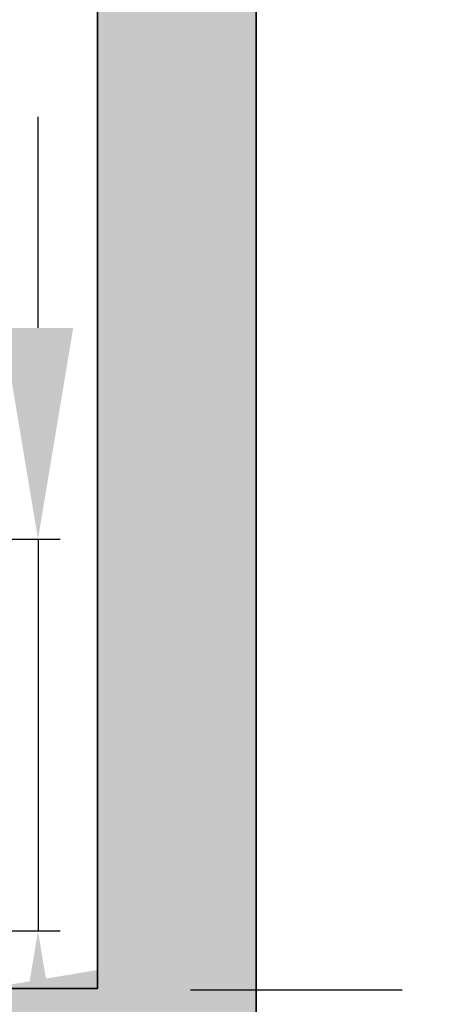
# Model space of a CAD drawing. Units: inches. Extents: x 2083 to 3317, y 1141 to 2115.
# Tile 240 of 256: x 3114 to 3137, y 1271 to 1327. Entities that reach past the tile are written whole.
import ezdxf

# ---------------------------------------------------------------- set-up
doc = ezdxf.new("R2010")
doc.units = ezdxf.units.IN
doc.layers.add('A-ANNO-DIMS', color=2, linetype='Continuous', lineweight=18)
doc.layers.add('A-WALL', color=7, linetype='Continuous', lineweight=35)
doc.layers.add('A-WALL-PATT', color=251, linetype='Continuous', lineweight=13, true_color=0x636466)
doc.styles.get("Standard").update_dxf_attribs({"font": 'arial.ttf'})
doc.dimstyles.new('ISO-25', dxfattribs={"dimtxt": 12, "dimasz": 12, "dimexe": 1.25, "dimexo": 0.625, "dimtad": 1, "dimlunit": 3, "dimtxsty": 'Standard', "dimcen": 2.5, "dimadec": 0, "dimazin": 0, "dimtfac": 1, "dimtmove": 0, "dimatfit": 3, "dimfxl": 1, "dimarcsym": 0})

# ---------------------------------------------------------------- blocks, each defined once
blk = doc.blocks.new('*D9')
at = {"layer": 'A-ANNO-DIMS', "color": 0, "lineweight": -2, "transparency": 16777216}
for p, q in [((3127.585, 1486.761), (3190.403, 1486.761)), ((3189.153, 1474.761), (3189.153, 1275.261)), ((3127.585, 1263.261), (3190.403, 1263.261))]:
    blk.add_line(p, q, dxfattribs=at)
at = {"layer": 'A-ANNO-DIMS', "color": 0, "transparency": 16777216}
for points in [[(3187.153, 1474.761), (3191.153, 1474.761), (3189.153, 1486.761)], [(3187.153, 1275.261), (3191.153, 1275.261), (3189.153, 1263.261)]]:
    blk.add_solid(points, dxfattribs=at)
at = {"layer": 'Defpoints', "color": 0, "transparency": 16777216}
for p in [(3126.96, 1486.761), (3126.96, 1263.261), (3189.153, 1263.261)]:
    blk.add_point(p, dxfattribs=at)
at = {"layer": 'A-ANNO-DIMS', "color": 0, "transparency": 16777216, "insert": (3182.401, 1375.011), "char_height": 12, "attachment_point": 5, "rotation": 90}
blk.add_mtext('18\'-7.5"', dxfattribs=at)
blk = doc.blocks.new('*D26')
at = {"layer": 'A-ANNO-DIMS', "color": 0, "lineweight": -2, "transparency": 16777216}
for p, q in [((3088.986, 1274.915), (3088.986, 1270.952)), ((3111.24, 1274.915), (3111.24, 1270.952)), ((3076.986, 1272.202), (2840.262, 1272.202)), ((3111.24, 1272.202), (3088.986, 1272.202)), ((3123.24, 1272.202), (3135.24, 1272.202))]:
    blk.add_line(p, q, dxfattribs=at)
at = {"layer": 'A-ANNO-DIMS', "color": 0, "transparency": 16777216}
for points in [[(3076.986, 1274.202), (3076.986, 1270.202), (3088.986, 1272.202)], [(3123.24, 1274.202), (3123.24, 1270.202), (3111.24, 1272.202)]]:
    blk.add_solid(points, dxfattribs=at)
at = {"layer": 'Defpoints', "color": 0, "transparency": 16777216}
for p in [(3088.986, 1275.54), (3111.24, 1275.54), (3088.986, 1272.202)]:
    blk.add_point(p, dxfattribs=at)
at = {"layer": 'A-ANNO-DIMS', "color": 0, "transparency": 16777216, "insert": (2952.624, 1279.032), "char_height": 12, "attachment_point": 5}
blk.add_mtext('NIGHTSTAND 1\'-10 1/2" TYP.', dxfattribs=at)
blk = doc.blocks.new('*D27')
at = {"layer": 'A-ANNO-DIMS', "color": 0, "lineweight": -2, "transparency": 16777216}
for p, q in [((3114.578, 1309.794), (3114.578, 1321.794)), ((3111.865, 1297.794), (3115.828, 1297.794)), ((3114.578, 1297.794), (3114.578, 1275.54)), ((3111.865, 1275.54), (3115.828, 1275.54)), ((3114.578, 1263.54), (3114.578, 1140.989))]:
    blk.add_line(p, q, dxfattribs=at)
at = {"layer": 'A-ANNO-DIMS', "color": 0, "transparency": 16777216}
for points in [[(3112.578, 1309.794), (3116.578, 1309.794), (3114.578, 1297.794)], [(3112.578, 1263.54), (3116.578, 1263.54), (3114.578, 1275.54)]]:
    blk.add_solid(points, dxfattribs=at)
at = {"layer": 'Defpoints', "color": 0, "transparency": 16777216}
for p in [(3111.24, 1297.794), (3111.24, 1275.54), (3114.578, 1275.54)]:
    blk.add_point(p, dxfattribs=at)
at = {"layer": 'A-ANNO-DIMS', "color": 0, "transparency": 16777216, "insert": (3107.749, 1196.264), "char_height": 12, "attachment_point": 5, "rotation": 90}
blk.add_mtext('1\'-10 1/2" TYP.', dxfattribs=at)
blk = doc.blocks.new('*D35')
at = {"layer": 'A-ANNO-DIMS', "color": 0, "lineweight": -2, "transparency": 16777216}
for p, q in [((3127.585, 2020.761), (3180.56, 2020.761)), ((3179.31, 1275.261), (3179.31, 2008.761)), ((3127.585, 1263.261), (3180.56, 1263.261))]:
    blk.add_line(p, q, dxfattribs=at)
at = {"layer": 'A-ANNO-DIMS', "color": 0, "transparency": 16777216}
for points in [[(3177.31, 2008.761), (3181.31, 2008.761), (3179.31, 2020.761)], [(3177.31, 1275.261), (3181.31, 1275.261), (3179.31, 1263.261)]]:
    blk.add_solid(points, dxfattribs=at)
at = {"layer": 'Defpoints', "color": 0, "transparency": 16777216}
for p in [(3126.96, 2020.761), (3179.31, 2020.761), (3126.96, 1263.261)]:
    blk.add_point(p, dxfattribs=at)
at = {"layer": 'A-ANNO-DIMS', "color": 0, "transparency": 16777216, "insert": (3172.476, 1642.011), "char_height": 12, "attachment_point": 5, "rotation": 90}
blk.add_mtext('63\'-1 1/2"', dxfattribs=at)

msp = doc.modelspace()

# ---------------------------------------------------------------- hatches: boundary and pattern name
at = {"layer": 'A-WALL-PATT'}
h = msp.add_hatch(color=256, dxfattribs=at)
h.dxf.hatch_style = 1
h.paths.add_polyline_path([(3126.96, 2020.761), (2748.96, 2020.761), (2604.96, 2020.761), (2226.96, 2020.761), (2226.96, 1702.761), (2466.96, 1702.761), (2466.96, 1582.761), (2418.96, 1582.761), (2418.96, 1477.761), (2226.96, 1477.761), (2226.96, 1263.261), (2544.96, 1263.261), (2544.96, 1411.761), (2604.96, 1411.761), (2685.96, 1411.761), (2685.96, 1420.761), (2604.96, 1420.761), (2604.96, 1573.761), (2604.96, 1702.761), (2604.96, 2011.761), (2748.96, 2011.761), (2748.96, 1702.761), (2862.96, 1702.761), (2862.96, 1621.761), (2871.96, 1621.761), (2871.96, 1702.761), (2883.96, 1702.761), (2883.96, 1706.939, -0.026459), (2883.96, 1711.761), (2757.96, 1711.761), (2757.96, 1807.761), (2787.96, 1807.761), (2787.96, 1812.261), (2757.96, 1812.261), (2757.96, 2011.761), (2877.96, 2011.761), (2877.96, 1812.261), (2847.96, 1812.261), (2847.96, 1807.761), (2889.836, 1807.761), (2889.836, 1812.261), (2882.46, 1812.261), (2882.46, 2011.761), (3117.96, 2011.761), (3117.96, 1812.261), (2937.836, 1812.261), (2937.836, 1807.761), (2995.71, 1807.761), (2995.71, 1796.118), (3000.21, 1796.118), (3000.21, 1807.761), (3117.96, 1807.761), (3117.96, 1711.761), (3000.21, 1711.761), (3000.21, 1760.118), (2998.573, 1760.118, -0.020711), (2995.71, 1760.118), (2995.71, 1711.761), (2931.96, 1711.761), (2931.96, 1702.761), (3126.96, 1702.761)])
h.paths.add_polyline_path([(2471.46, 2011.761), (2471.46, 1810.011), (2462.717, 1810.011), (2462.717, 1805.511), (2505.96, 1805.511), (2505.96, 1810.011), (2475.96, 1810.011), (2475.96, 2011.761), (2595.96, 2011.761), (2595.96, 1810.011), (2565.96, 1810.011), (2565.96, 1805.511), (2595.96, 1805.511), (2595.96, 1711.761), (2235.96, 1711.761), (2235.96, 1805.511), (2353.71, 1805.511), (2353.71, 1796.054), (2358.21, 1796.054), (2358.21, 1805.511), (2414.717, 1805.511), (2414.717, 1810.011), (2235.96, 1810.011), (2235.96, 2011.761)], flags=16)
h.paths.add_polyline_path([(2270.205, 1994.61), (2270.205, 1970.61), (2246.205, 1970.61), (2246.205, 1994.61)], flags=0)
edge = h.paths.add_edge_path(flags=0)
edge.add_ellipse((2332.027, 1899.798), major_axis=(-3.043, 3.043), ratio=0.168252, start_angle=-161.3322, end_angle=-156.3071, ccw=False)
edge.add_ellipse((2333.082, 1898.744), major_axis=(-1.055, 1.055), ratio=0.453532, start_angle=-123.371, end_angle=-94.1591)
edge = h.paths.add_edge_path(flags=0)
edge.add_ellipse((2332.027, 1968.876), major_axis=(3.043, 3.043), ratio=0.168252, start_angle=18.6678, end_angle=23.6929)
edge.add_spline(control_points=[(2332.926, 1970.691), (2332.227, 1970.336), (2330.894, 1969.659), (2328.413, 1970.932), (2327.204, 1967.749), (2324.71, 1969.956), (2322.533, 1967.012), (2320.013, 1971.296), (2317.68, 1968.158), (2316.041, 1967.102), (2315.427, 1966.81)], knot_values=[0, 0, 0, 0, 2.267059, 4.324559, 6.685584, 8.878641, 11.121502, 14.300359, 17.755284, 19.732645, 19.732645, 19.732645, 19.732645], degree=3, periodic=0)
edge.add_ellipse((2332.027, 1968.876), major_axis=(3.043, 3.043), ratio=0.168252, start_angle=18.6678, end_angle=23.6929, ccw=False)
edge.add_ellipse((2333.082, 1969.931), major_axis=(1.055, 1.055), ratio=0.453532, start_angle=56.629, end_angle=85.8409, ccw=False)
edge = h.paths.add_edge_path(flags=0)
edge.add_spline(control_points=[(2296.428, 1967.988), (2293.628, 1965.336), (2287.704, 1959.727), (2299.744, 1949.996), (2294.533, 1935.669), (2290.573, 1920.604), (2293.394, 1909.974), (2296.185, 1904.967)], knot_values=[0.099185, 0.099185, 0.099185, 0.099185, 0.345301, 0.619822, 0.982653, 1.386093, 1.810555, 1.810555, 1.810555, 1.810555], degree=3, periodic=0)
edge.add_spline(control_points=[(2296.185, 1904.967), (2297.384, 1902.619), (2298.001, 1901.949), (2298.553, 1901.468)], knot_values=[0.006246, 0.006246, 0.006246, 0.006246, 0.055476, 0.055476, 0.055476, 0.055476], degree=3, periodic=0)
edge.add_spline(control_points=[(2298.553, 1901.468), (2297.259, 1900.923), (2295.225, 1900.232), (2293.06, 1900.614), (2292.101, 1900.788), (2292.09, 1900.791)], knot_values=[0.312835, 0.312835, 0.312835, 0.312835, 0.40178, 0.474987, 0.475903, 0.475903, 0.475903, 0.475903], degree=3, periodic=0)
edge.add_arc((2292.794, 1904.664), 3.937, 215.4209, 259.6982, ccw=False)
edge.add_spline(control_points=[(2289.585, 1902.382), (2289.477, 1902.535), (2289.368, 1902.688), (2289.261, 1902.841)], knot_values=[0.102872, 0.102872, 0.102872, 0.102872, 0.116896, 0.116896, 0.116896, 0.116896], degree=3, periodic=0)
edge.add_spline(control_points=[(2289.261, 1902.841), (2288.687, 1902.55), (2287.64, 1902.02), (2285.881, 1901.874), (2283.853, 1901.504), (2281.72, 1899.711), (2278.467, 1899.493), (2276.157, 1901.883), (2272.259, 1899.804), (2267.778, 1901.843), (2262.244, 1900.184), (2257.415, 1901.782), (2254.318, 1900.726), (2253.178, 1900.337)], knot_values=[0, 0, 0, 0, 1.907977, 3.477176, 5.261074, 7.972851, 11.680248, 13.717921, 16.939592, 22.789562, 27.502503, 33.595215, 37.145618, 37.145618, 37.145618, 37.145618], degree=3, periodic=0)
edge.add_line((2253.178, 1900.337), (2250.244, 1902.841))
edge.add_line((2250.244, 1902.841), (2250.244, 1965.833))
edge.add_line((2250.244, 1965.833), (2253.178, 1968.337))
edge.add_spline(control_points=[(2253.178, 1968.337), (2254.318, 1967.948), (2257.415, 1966.892), (2262.244, 1968.49), (2267.778, 1966.831), (2271.527, 1968.537), (2273.876, 1967.828), (2274.207, 1967.728)], knot_values=[0, 0, 0, 0, 0.09018, 0.244935, 0.364644, 0.513233, 0.537855, 0.537855, 0.537855, 0.537855], degree=3, periodic=0)
edge.add_arc((2274.353, 1963.793), 3.937, 72.0511, 92.1279, ccw=False)
edge.add_arc((2281.297, 1985.23), 18.596, 252.0511, 288.5657)
edge.add_arc((2292.317, 1956.029), 12.646, 71.0268, 113.7782, ccw=False)
edge = h.paths.add_edge_path(flags=0)
edge.add_spline(control_points=[(2274.899, 1951.856), (2275.066, 1951.617), (2275.233, 1951.377), (2275.398, 1951.136)], knot_values=[1.409916, 1.409916, 1.409916, 1.409916, 1.43159, 1.43159, 1.43159, 1.43159], degree=3, periodic=0)
edge.add_spline(control_points=[(2275.398, 1951.136), (2275.792, 1950.562), (2276.179, 1949.984), (2276.546, 1949.397)], knot_values=[1.358238, 1.358238, 1.358238, 1.358238, 1.409916, 1.409916, 1.409916, 1.409916], degree=3, periodic=0)
edge.add_line((2276.546, 1949.397), (2277.437, 1947.862))
edge.add_spline(control_points=[(2277.437, 1947.862), (2276.304, 1945.673), (2274.64, 1942.427), (2274.632, 1938.094), (2272.799, 1930.852), (2274.356, 1943.897), (2275.948, 1947.923), (2276.546, 1949.397)], knot_values=[0.005632, 0.005632, 0.005632, 0.005632, 0.186014, 0.266002, 0.357087, 0.59639, 0.739732, 0.739732, 0.739732, 0.739732], degree=3, periodic=0)
edge.add_spline(control_points=[(2276.546, 1949.397), (2276.179, 1949.984), (2275.792, 1950.562), (2275.398, 1951.136)], knot_values=[1.358238, 1.358238, 1.358238, 1.358238, 1.409916, 1.409916, 1.409916, 1.409916], degree=3, periodic=0)
edge.add_spline(control_points=[(2275.398, 1951.136), (2274.943, 1950.08), (2274.208, 1948.025), (2273.935, 1944.851), (2272.469, 1937.627), (2273.466, 1945.696), (2274.701, 1951.059), (2274.899, 1951.856)], knot_values=[0.104364, 0.104364, 0.104364, 0.104364, 0.189636, 0.269624, 0.36071, 0.600013, 0.644622, 0.644622, 0.644622, 0.644622], degree=3, periodic=0)
h.paths.add_polyline_path([(2269.168, 1963.128, -0.357527), (2268.171, 1960.976, -0.092561), (2268.171, 1939.436, -0.357527), (2269.168, 1937.285, -0.357527), (2267.016, 1938.282, -0.164785), (2254.686, 1938.282, -0.357527), (2252.534, 1937.285, -0.357527), (2253.531, 1939.436, -0.092561), (2253.531, 1960.976, -0.357527), (2252.534, 1963.128, -0.357527), (2254.686, 1962.131, -0.164785), (2267.016, 1962.131, -0.357527)], flags=0)
h.paths.add_polyline_path([(2248.874, 1967.802), (2248.874, 1957.028), (2249.458, 1957.028), (2249.458, 1911.647), (2248.874, 1911.647), (2248.874, 1900.873), (2246.512, 1900.873, 0.197327), (2244.15, 1902.457), (2244.15, 1966.218, 0.197327), (2246.512, 1967.802)], flags=0)
h.paths.add_polyline_path([(2269.168, 1931.389, -0.357527), (2268.171, 1929.238, -0.092561), (2268.171, 1907.698, -0.357527), (2269.168, 1905.547, -0.357527), (2267.016, 1906.544, -0.164785), (2254.686, 1906.544, -0.357527), (2252.534, 1905.547, -0.357527), (2253.531, 1907.698, -0.092561), (2253.531, 1929.238, -0.357527), (2252.534, 1931.389, -0.357527), (2254.686, 1930.392, -0.164785), (2267.016, 1930.392, -0.357527)], flags=0)
edge = h.paths.add_edge_path(flags=0)
edge.add_spline(control_points=[(2276.197, 1906.724), (2276.168, 1909.029), (2276.114, 1913.372), (2270.598, 1924.925), (2273.905, 1919.013), (2275.922, 1916.262), (2275.475, 1912.402), (2277.258, 1910.381), (2276.696, 1908.225), (2276.646, 1906.813), (2276.618, 1906.008)], knot_values=[0, 0, 0, 0, 8.61026, 16.221274, 18.843057, 23.804898, 27.440828, 29.356102, 31.203478, 33.650687, 33.650687, 33.650687, 33.650687], degree=3, periodic=0)
edge.add_spline(control_points=[(2276.618, 1906.008), (2276.623, 1905.624), (2276.498, 1904.629), (2275.442, 1903.855), (2274.937, 1903.08), (2274.859, 1902.841)], knot_values=[0.156488, 0.156488, 0.156488, 0.156488, 0.184398, 0.231376, 0.250598, 0.250598, 0.250598, 0.250598], degree=3, periodic=0)
edge.add_line((2274.859, 1902.841), (2276.506, 1902.841))
edge.add_spline(control_points=[(2276.506, 1902.841), (2276.788, 1903.085), (2277.665, 1904.125), (2278.25, 1904.341), (2277.654, 1908.527), (2278.156, 1906.228), (2278.1, 1905.286), (2278.847, 1904.069), (2277.857, 1903.415), (2277.874, 1902.991), (2277.904, 1902.841)], knot_values=[0.059574, 0.059574, 0.059574, 0.059574, 0.080753, 0.103741, 0.16972, 0.176036, 0.207137, 0.240474, 0.262341, 0.27366, 0.27366, 0.27366, 0.27366], degree=3, periodic=0)
edge.add_line((2277.904, 1902.841), (2280.03, 1902.841))
edge.add_spline(control_points=[(2280.03, 1902.841), (2279.888, 1903.088), (2279.499, 1903.982), (2280.152, 1905.939), (2278.104, 1909.658), (2279.762, 1907.185), (2280.328, 1904.875), (2280.485, 1903.49), (2281.463, 1903.249), (2281.758, 1902.936), (2281.834, 1902.841)], knot_values=[0.013856, 0.013856, 0.013856, 0.013856, 0.034874, 0.088867, 0.107879, 0.126738, 0.158714, 0.193757, 0.217487, 0.226722, 0.226722, 0.226722, 0.226722], degree=3, periodic=0)
edge.add_spline(control_points=[(2281.834, 1902.841), (2281.788, 1902.827), (2281.647, 1902.783), (2281.396, 1902.859), (2281.088, 1902.985), (2280.721, 1903.061), (2280.333, 1903.026), (2280.125, 1902.899), (2280.03, 1902.841)], knot_values=[0, 0, 0, 0, 0.14413, 0.435517, 0.749276, 1.153046, 1.548371, 1.878348, 1.878348, 1.878348, 1.878348], degree=3, periodic=0)
edge.add_line((2280.03, 1902.841), (2277.904, 1902.841))
edge.add_spline(control_points=[(2277.904, 1902.841), (2277.893, 1902.796), (2277.865, 1902.68), (2277.607, 1902.687), (2277.274, 1902.801), (2276.838, 1902.62), (2276.584, 1902.789), (2276.506, 1902.841)], knot_values=[0, 0, 0, 0, 0.127189, 0.326199, 0.628009, 1.24357, 1.515331, 1.515331, 1.515331, 1.515331], degree=3, periodic=0)
edge.add_line((2276.506, 1902.841), (2274.859, 1902.841))
edge.add_spline(control_points=[(2274.859, 1902.841), (2274.814, 1902.899), (2274.725, 1903.013), (2274.493, 1903.119), (2274.244, 1902.961), (2273.937, 1903.185), (2273.614, 1902.983), (2273.408, 1902.883), (2273.322, 1902.841)], knot_values=[0, 0, 0, 0, 0.21843, 0.436957, 0.687977, 0.990379, 1.398396, 1.69185, 1.69185, 1.69185, 1.69185], degree=3, periodic=0)
edge.add_spline(control_points=[(2273.322, 1902.841), (2273.617, 1903.446), (2274.274, 1904.538), (2276.027, 1904.574), (2276.207, 1906.584), (2276.197, 1906.724)], knot_values=[0.012227, 0.012227, 0.012227, 0.012227, 0.059472, 0.106218, 0.134458, 0.134458, 0.134458, 0.134458], degree=3, periodic=0)
h.paths.add_polyline_path([(2270.776, 1897.79), (2270.776, 1873.79), (2246.776, 1873.79), (2246.776, 1897.79)], flags=0)
h.paths.add_polyline_path([(2353.71, 1760.005), (2353.71, 1760.054), (2358.21, 1760.054, -0.033729)], flags=0)
h.paths.add_polyline_path([(2321.819, 1737.529), (2341.995, 1737.529, -0.414214), (2343.203, 1736.321), (2343.203, 1721.021, -0.414214), (2341.995, 1719.813), (2321.819, 1719.813, -0.414214), (2320.611, 1721.021), (2320.611, 1736.321, -0.414214)], flags=0)
h.paths.add_polyline_path([(2324.235, 1736.321), (2339.579, 1736.321, -0.414214), (2341.995, 1733.905), (2341.995, 1725.45, -0.414214), (2339.579, 1723.034), (2333.681, 1723.034), (2333.845, 1722.045, -0.870646), (2335.425, 1721.826, -0.767327), (2333.923, 1721.423), (2331.291, 1721.423, -0.767327), (2329.788, 1721.826, -0.870646), (2331.368, 1722.045), (2331.533, 1723.034), (2324.235, 1723.034, -0.414214), (2321.819, 1725.45), (2321.819, 1733.905, -0.414214)], flags=0)
h.paths.add_polyline_path([(2570.484, 1928.615), (2589.684, 1928.615), (2590.169, 1928.615), (2590.169, 1904.993), (2570.484, 1904.993)], flags=0)
h.paths.add_polyline_path([(2574.447, 1927.264, -1), (2572.829, 1927.264, -1)], flags=0)
h.paths.add_polyline_path([(2573.09, 1926.941), (2573.925, 1927.776), (2574.148, 1927.553), (2573.313, 1926.718)], flags=0)
h.paths.add_polyline_path([(2578.779, 1919.73, -1), (2571.592, 1919.73, -1)], flags=0)
h.paths.add_polyline_path([(2578.385, 1919.73, -1), (2571.985, 1919.73, -1)], flags=0)
h.paths.add_polyline_path([(2331.596, 1729.476, -1), (2333.618, 1729.476, -1)], flags=0)
h.paths.add_polyline_path([(2578.034, 1927.264, -1), (2576.416, 1927.264, -1)], flags=0)
h.paths.add_polyline_path([(2576.689, 1927.531), (2576.912, 1927.754), (2577.747, 1926.919), (2577.524, 1926.696)], flags=0)
h.paths.add_polyline_path([(2578.139, 1909.86, -1), (2572.232, 1909.86, -1)], flags=0)
h.paths.add_polyline_path([(2577.745, 1909.86, -1), (2572.625, 1909.86, -1)], flags=0)
h.paths.add_polyline_path([(2583.798, 1927.264, -1), (2582.179, 1927.264, -1)], flags=0)
h.paths.add_polyline_path([(2582.719, 1927.754), (2583.554, 1926.919), (2583.331, 1926.696), (2582.496, 1927.531)], flags=0)
h.paths.add_polyline_path([(2582.496, 1927.531), (2582.719, 1927.754), (2583.554, 1926.919), (2583.331, 1926.696)], flags=0)
h.paths.add_polyline_path([(2587.739, 1920.53, -1), (2581.832, 1920.53, -1)], flags=0)
h.paths.add_polyline_path([(2587.345, 1920.53, -1), (2582.225, 1920.53, -1)], flags=0)
h.paths.add_polyline_path([(2587.385, 1927.264, -1), (2585.766, 1927.264, -1)], flags=0)
h.paths.add_polyline_path([(2586.082, 1926.98), (2586.917, 1927.815), (2587.14, 1927.593), (2586.305, 1926.758)], flags=0)
h.paths.add_polyline_path([(2588.379, 1910.66, -1), (2581.192, 1910.66, -1)], flags=0)
h.paths.add_polyline_path([(2587.985, 1910.66, -1), (2581.585, 1910.66, -1)], flags=0)
h.paths.add_polyline_path([(2417.168, 1729.478), (2437.344, 1729.478, -0.414214), (2438.552, 1728.27), (2438.552, 1712.969, -0.414214), (2437.344, 1711.761), (2417.168, 1711.761, -0.414214), (2415.96, 1712.969), (2415.96, 1728.27, -0.414214)], flags=0)
h.paths.add_polyline_path([(2419.584, 1728.27), (2434.928, 1728.27, -0.414214), (2437.344, 1725.854), (2437.344, 1717.398, -0.414214), (2434.928, 1714.983), (2429.029, 1714.983), (2429.194, 1713.994, -0.870646), (2430.774, 1713.775, -0.767327), (2429.271, 1713.372), (2426.64, 1713.372, -0.767327), (2425.137, 1713.775, -0.870646), (2426.717, 1713.994), (2426.882, 1714.983), (2419.584, 1714.983, -0.414214), (2417.168, 1717.398), (2417.168, 1725.854, -0.414214)], flags=0)
h.paths.add_polyline_path([(2419.584, 1728.27), (2434.928, 1728.27, -0.414214), (2437.344, 1725.854), (2437.344, 1717.398, -0.414214), (2434.928, 1714.983), (2429.029, 1714.983), (2428.358, 1719.009), (2427.553, 1719.009), (2426.882, 1714.983), (2419.584, 1714.983, -0.414214), (2417.168, 1717.398), (2417.168, 1725.854, -0.414214)], flags=0)
h.paths.add_polyline_path([(2426.944, 1721.425, -1), (2428.967, 1721.425, -1)], flags=0)
h.paths.add_polyline_path([(2475.96, 1702.761), (2595.96, 1702.761), (2595.96, 1582.761), (2475.96, 1582.761)], flags=16)
h.paths.add_polyline_path([(2427.96, 1573.761), (2595.96, 1573.761), (2595.96, 1468.761), (2595.96, 1420.761), (2384.46, 1420.761), (2384.46, 1468.761), (2427.96, 1468.761)], flags=16)
h.paths.add_polyline_path([(2379.96, 1468.761), (2379.96, 1420.761), (2235.96, 1420.761), (2235.96, 1468.761)], flags=16)
h.paths.add_polyline_path([(2317.816, 1466.696), (2337.992, 1466.696, -0.414214), (2339.2, 1465.488), (2339.2, 1450.187, -0.414214), (2337.992, 1448.979), (2317.816, 1448.979, -0.414214), (2316.608, 1450.187), (2316.608, 1465.488, -0.414214)], flags=0)
h.paths.add_polyline_path([(2320.232, 1465.488), (2335.576, 1465.488, -0.414214), (2337.992, 1463.072), (2337.992, 1454.616, -0.414214), (2335.576, 1452.2), (2329.677, 1452.2), (2329.842, 1451.212, -0.870646), (2331.422, 1450.992, -0.767327), (2329.92, 1450.59), (2327.288, 1450.59, -0.767327), (2325.785, 1450.992, -0.870646), (2327.365, 1451.212), (2327.53, 1452.2), (2320.232, 1452.2, -0.414214), (2317.816, 1454.616), (2317.816, 1463.072, -0.414214)], flags=0)
h.paths.add_polyline_path([(2320.232, 1465.488), (2335.576, 1465.488, -0.414214), (2337.992, 1463.072), (2337.992, 1454.616, -0.414214), (2335.576, 1452.2), (2329.677, 1452.2), (2329.006, 1456.227), (2328.201, 1456.227), (2327.53, 1452.2), (2320.232, 1452.2, -0.414214), (2317.816, 1454.616), (2317.816, 1463.072, -0.414214)], flags=0)
h.paths.add_polyline_path([(2327.593, 1458.643, -1), (2329.615, 1458.643, -1)], flags=0)
h.paths.add_polyline_path([(2244.412, 1433.34), (2241.921, 1433.34, -0.414214), (2240.018, 1435.244), (2240.018, 1440.953, -0.414211), (2241.921, 1442.856), (2244.412, 1442.856, -1.976472)], flags=0)
h.paths.add_polyline_path([(2245.357, 1434.398, -0.414214), (2245.357, 1441.799, -2.144098)], flags=0)
h.paths.add_polyline_path([(2535.96, 1416.261), (2535.96, 1272.261), (2235.96, 1272.261), (2235.96, 1416.261)], flags=16)
h.paths.add_polyline_path([(2260.12, 1384.293), (2260.12, 1362.039), (2237.865, 1362.039), (2237.865, 1384.293)], flags=0)
edge = h.paths.add_edge_path(flags=0)
edge.add_line((2318.252, 1362.093), (2318.146, 1362.001))
edge.add_ellipse((2317.445, 1360.431), major_axis=(2.822, 2.822), ratio=0.168252, start_angle=18.6678, end_angle=20.9481, ccw=False)
edge.add_ellipse((2318.423, 1361.409), major_axis=(0.978, 0.978), ratio=0.453532, start_angle=56.629, end_angle=70.2262, ccw=False)
edge = h.paths.add_edge_path(flags=0)
edge.add_line((2319.107, 1295.571), (2319.015, 1295.677))
edge.add_ellipse((2317.445, 1296.378), major_axis=(-2.822, 2.822), ratio=0.168252, start_angle=-161.3322, end_angle=-159.0519, ccw=False)
edge.add_ellipse((2318.423, 1295.4), major_axis=(-0.978, 0.978), ratio=0.453532, start_angle=-123.371, end_angle=-109.7738)
edge = h.paths.add_edge_path(flags=0)
edge.add_spline(control_points=[(2284.21, 1301.17), (2284.581, 1300.445), (2284.891, 1299.892), (2285.16, 1299.461)], knot_values=[0.039066, 0.039066, 0.039066, 0.039066, 0.055476, 0.055476, 0.055476, 0.055476], degree=3, periodic=0)
edge.add_line((2285.16, 1299.461), (2284.21, 1301.17))
edge = h.paths.add_edge_path(flags=0)
edge.add_line((2280.412, 1297.298), (2283.37, 1297.036))
edge.add_line((2283.37, 1297.036), (2286.406, 1297.926))
edge.add_spline(control_points=[(2286.406, 1297.926), (2285.305, 1297.463), (2284.345, 1297.129), (2283.37, 1297.036)], knot_values=[0.394369, 0.394369, 0.394369, 0.394369, 0.475903, 0.475903, 0.475903, 0.475903], degree=3, periodic=0)
edge.add_spline(control_points=[(2283.37, 1297.036), (2283.281, 1297.028), (2282.316, 1296.957), (2281.313, 1297.134), (2280.423, 1297.296), (2280.412, 1297.298)], knot_values=[0.312835, 0.312835, 0.312835, 0.312835, 0.320246, 0.393453, 0.394369, 0.394369, 0.394369, 0.394369], degree=3, periodic=0)
edge = h.paths.add_edge_path(flags=0)
edge.add_line((2284.436, 1359.607), (2280.446, 1355.328))
edge.add_line((2280.446, 1355.328), (2279.58, 1351.018))
edge.add_line((2279.58, 1351.018), (2282.413, 1346.58))
edge.add_spline(control_points=[(2282.413, 1346.58), (2283.153, 1345.589), (2284.253, 1344.029), (2284.801, 1342.387), (2284.935, 1341.806)], knot_values=[1.240098, 1.240098, 1.240098, 1.240098, 1.332892, 1.382712, 1.382712, 1.382712, 1.382712], degree=3, periodic=0)
edge.add_spline(control_points=[(2284.935, 1341.806), (2285.319, 1340.141), (2285.233, 1338.409), (2284.91, 1336.654)], knot_values=[1.097484, 1.097484, 1.097484, 1.097484, 1.240098, 1.240098, 1.240098, 1.240098], degree=3, periodic=0)
edge.add_spline(control_points=[(2284.91, 1336.654), (2284.587, 1334.899), (2284.027, 1333.12), (2283.463, 1331.361)], knot_values=[0.95487, 0.95487, 0.95487, 0.95487, 1.097484, 1.097484, 1.097484, 1.097484], degree=3, periodic=0)
edge.add_line((2283.463, 1331.361), (2281.89, 1326.153))
edge.add_line((2281.89, 1326.153), (2280.756, 1321.056))
edge.add_line((2280.756, 1321.056), (2280.299, 1316.002))
edge.add_line((2280.299, 1316.002), (2280.716, 1310.95))
edge.add_line((2280.716, 1310.95), (2282.028, 1305.972))
edge.add_line((2282.028, 1305.972), (2284.21, 1301.17))
edge.add_spline(control_points=[(2284.21, 1301.17), (2283.341, 1302.73), (2282.612, 1304.336), (2282.028, 1305.972)], knot_values=[0.099185, 0.099185, 0.099185, 0.099185, 0.241799, 0.241799, 0.241799, 0.241799], degree=3, periodic=0)
edge.add_spline(control_points=[(2282.028, 1305.972), (2281.444, 1307.608), (2281.005, 1309.273), (2280.716, 1310.95)], knot_values=[0.241799, 0.241799, 0.241799, 0.241799, 0.384413, 0.384413, 0.384413, 0.384413], degree=3, periodic=0)
edge.add_spline(control_points=[(2280.716, 1310.95), (2280.433, 1312.588), (2280.289, 1314.277), (2280.299, 1315.962), (2280.299, 1316.002)], knot_values=[0.384413, 0.384413, 0.384413, 0.384413, 0.523647, 0.527028, 0.527028, 0.527028, 0.527028], degree=3, periodic=0)
edge.add_spline(control_points=[(2280.299, 1316.002), (2280.312, 1317.687), (2280.478, 1319.368), (2280.756, 1321.056)], knot_values=[0.527028, 0.527028, 0.527028, 0.527028, 0.669642, 0.669642, 0.669642, 0.669642], degree=3, periodic=0)
edge.add_spline(control_points=[(2280.756, 1321.056), (2281.035, 1322.744), (2281.426, 1324.44), (2281.89, 1326.153)], knot_values=[0.669642, 0.669642, 0.669642, 0.669642, 0.812256, 0.812256, 0.812256, 0.812256], degree=3, periodic=0)
edge.add_spline(control_points=[(2281.89, 1326.153), (2282.264, 1327.533), (2282.788, 1329.262), (2283.353, 1331.018), (2283.463, 1331.361)], knot_values=[0.812256, 0.812256, 0.812256, 0.812256, 0.927087, 0.95487, 0.95487, 0.95487, 0.95487], degree=3, periodic=0)
edge.add_line((2283.463, 1331.361), (2284.91, 1336.654))
edge.add_line((2284.91, 1336.654), (2284.935, 1341.806))
edge.add_line((2284.935, 1341.806), (2282.413, 1346.58))
edge.add_spline(control_points=[(2282.413, 1346.58), (2281.275, 1348.104), (2280.078, 1349.57), (2279.58, 1351.018)], knot_values=[1.382712, 1.382712, 1.382712, 1.382712, 1.525326, 1.525326, 1.525326, 1.525326], degree=3, periodic=0)
edge.add_spline(control_points=[(2279.58, 1351.018), (2279.443, 1351.415), (2279.136, 1352.857), (2279.735, 1354.29), (2280.446, 1355.328)], knot_values=[1.525326, 1.525326, 1.525326, 1.525326, 1.564439, 1.667941, 1.667941, 1.667941, 1.667941], degree=3, periodic=0)
edge.add_spline(control_points=[(2280.446, 1355.328), (2281.426, 1356.758), (2282.931, 1358.183), (2284.436, 1359.607)], knot_values=[1.667941, 1.667941, 1.667941, 1.667941, 1.810555, 1.810555, 1.810555, 1.810555], degree=3, periodic=0)
edge.add_arc((2280.623, 1348.518), 11.726, 71.0268, 113.7782)
edge.add_arc((2270.405, 1375.595), 17.244, 252.0511, 288.5657, ccw=False)
edge.add_arc((2263.966, 1355.718), 3.651, 72.0511, 92.1279)
edge.add_arc((2263.966, 1355.718), 3.651, 92.1279, 177.9851)
edge.add_spline(control_points=[(2260.318, 1355.846), (2260.26, 1354.221), (2260.551, 1350.187), (2262.999, 1346.766), (2264.473, 1344.649)], knot_values=[1.43159, 1.43159, 1.43159, 1.43159, 1.564144, 1.770695, 1.770695, 1.770695, 1.770695], degree=3, periodic=0)
edge.add_line((2264.473, 1344.649), (2264.936, 1343.983))
edge.add_spline(control_points=[(2263.801, 1340.248), (2263.843, 1340.514), (2264.067, 1341.756), (2264.513, 1343.002), (2264.935, 1343.981)], knot_values=[0.53657, 0.53657, 0.53657, 0.53657, 0.559349, 0.644622, 0.644622, 0.644622, 0.644622], degree=3, periodic=0)
edge.add_spline(control_points=[(2264.935, 1343.981), (2265.118, 1343.715), (2265.299, 1343.448), (2265.477, 1343.179)], knot_values=[1.384077, 1.384077, 1.384077, 1.384077, 1.409916, 1.409916, 1.409916, 1.409916], degree=3, periodic=0)
edge.add_spline(control_points=[(2265.477, 1343.179), (2265.655, 1342.911), (2265.829, 1342.641), (2265.999, 1342.369)], knot_values=[1.358238, 1.358238, 1.358238, 1.358238, 1.384077, 1.384077, 1.384077, 1.384077], degree=3, periodic=0)
edge.add_line((2265.999, 1342.369), (2266.826, 1340.946))
edge.add_spline(control_points=[(2266.826, 1340.946), (2268.894, 1337.09), (2271.398, 1325.843), (2270.516, 1310.569), (2275.919, 1301.861), (2277.79, 1299.199)], knot_values=[0.116896, 0.116896, 0.116896, 0.116896, 0.472987, 1.050969, 1.313793, 1.313793, 1.313793, 1.313793], degree=3, periodic=0)
edge.add_spline(control_points=[(2277.79, 1299.199), (2277.839, 1299.128), (2277.889, 1299.057), (2277.94, 1298.987)], knot_values=[0.109884, 0.109884, 0.109884, 0.109884, 0.116896, 0.116896, 0.116896, 0.116896], degree=3, periodic=0)
edge.add_line((2277.94, 1298.987), (2277.789, 1299.199))
edge.add_spline(control_points=[(2277.789, 1299.199), (2277.257, 1298.929), (2276.286, 1298.438), (2275.039, 1298.334), (2274.383, 1298.239), (2274.215, 1298.209)], knot_values=[33.12187, 33.12187, 33.12187, 33.12187, 35.029056, 36.598255, 37.144827, 37.144827, 37.144827, 37.144827], degree=3, periodic=0)
edge.add_line((2274.215, 1298.209), (2273.073, 1297.893))
edge.add_spline(control_points=[(2273.073, 1297.893), (2272.323, 1297.58), (2271.039, 1296.511), (2269.248, 1296.226), (2268.423, 1296.375)], knot_values=[26.532584, 26.532584, 26.532584, 26.532584, 29.198919, 31.839101, 31.839101, 31.839101, 31.839101], degree=3, periodic=0)
edge.add_line((2268.423, 1296.375), (2263.879, 1297.458))
edge.add_spline(control_points=[(2263.879, 1297.458), (2263.556, 1297.359), (2261.86, 1296.839), (2260.239, 1297.282), (2258.933, 1297.516)], knot_values=[15.919551, 15.919551, 15.919551, 15.919551, 16.939592, 21.226067, 21.226067, 21.226067, 21.226067], degree=3, periodic=0)
edge.add_line((2258.933, 1297.516), (2254.055, 1297.329))
edge.add_spline(control_points=[(2254.055, 1297.329), (2253.756, 1297.296), (2252.114, 1297.165), (2250.462, 1297.544), (2249.13, 1297.668)], knot_values=[5.306517, 5.306517, 5.306517, 5.306517, 6.276435, 10.613034, 10.613034, 10.613034, 10.613034], degree=3, periodic=0)
edge.add_line((2249.13, 1297.668), (2244.332, 1296.878))
edge.add_line((2244.332, 1296.878), (2241.611, 1299.199))
edge.add_line((2241.611, 1299.199), (2241.611, 1357.609))
edge.add_line((2241.611, 1357.609), (2244.332, 1359.931))
edge.add_line((2244.332, 1359.931), (2252.729, 1359.543))
edge.add_spline(control_points=[(2252.729, 1359.543), (2252.871, 1359.546), (2253.306, 1359.548), (2253.74, 1359.514), (2254.032, 1359.482)], knot_values=[0.233291, 0.233291, 0.233291, 0.233291, 0.244935, 0.268927, 0.268927, 0.268927, 0.268927], degree=3, periodic=0)
edge.add_line((2254.032, 1359.482), (2259.587, 1359.416))
edge.add_spline(control_points=[(2259.587, 1359.416), (2260.677, 1359.629), (2262.073, 1359.897), (2263.524, 1359.459), (2263.83, 1359.366)], knot_values=[0.422516, 0.422516, 0.422516, 0.422516, 0.513233, 0.537855, 0.537855, 0.537855, 0.537855], degree=3, periodic=0)
edge.add_arc((2263.966, 1355.718), 3.651, 72.0511, 92.1279, ccw=False)
edge.add_arc((2270.405, 1375.595), 17.244, 252.0511, 288.5657)
edge.add_arc((2280.623, 1348.518), 11.726, 71.0268, 113.7782, ccw=False)
h.paths.add_polyline_path([(2240.341, 1359.435), (2240.341, 1349.444), (2240.882, 1349.444), (2240.882, 1307.365), (2240.341, 1307.365), (2240.341, 1297.374), (2238.15, 1297.374, 0.197327), (2235.96, 1298.843), (2235.96, 1357.966, 0.197327), (2238.15, 1359.435)], flags=0)
h.paths.add_polyline_path([(2259.158, 1355.101, -0.357527), (2258.233, 1353.106, -0.092561), (2258.233, 1333.133, -0.357527), (2259.158, 1331.138, -0.357527), (2257.163, 1332.062, -0.164785), (2245.729, 1332.062, -0.357527), (2243.735, 1331.138, -0.357527), (2244.659, 1333.133, -0.092561), (2244.659, 1353.106, -0.357527), (2243.735, 1355.101, -0.357527), (2245.729, 1354.176, -0.164785), (2257.163, 1354.176, -0.357527)], flags=0)
edge = h.paths.add_edge_path(flags=0)
edge.add_line((2265.999, 1342.369), (2266.826, 1340.946))
edge.add_line((2266.826, 1340.946), (2265.308, 1337.814))
edge.add_line((2265.308, 1337.814), (2264.358, 1334.653))
edge.add_line((2264.358, 1334.653), (2264.262, 1333.8))
edge.add_spline(control_points=[(2264.262, 1333.8), (2264.208, 1333.187), (2264.162, 1332.366), (2264.007, 1331.414), (2263.969, 1331.202)], knot_values=[0.464444, 0.464444, 0.464444, 0.464444, 0.516691, 0.531608, 0.531608, 0.531608, 0.531608], degree=3, periodic=0)
edge.add_spline(control_points=[(2263.969, 1331.202), (2263.775, 1330.119), (2263.424, 1328.791), (2263.257, 1328.531), (2263.234, 1328.515)], knot_values=[0.372682, 0.372682, 0.372682, 0.372682, 0.44885, 0.464444, 0.464444, 0.464444, 0.464444], degree=3, periodic=0)
edge.add_spline(control_points=[(2263.234, 1328.515), (2263.096, 1328.42), (2263.131, 1329.301), (2263.275, 1330.616)], knot_values=[0.280919, 0.280919, 0.280919, 0.280919, 0.372682, 0.372682, 0.372682, 0.372682], degree=3, periodic=0)
edge.add_spline(control_points=[(2263.275, 1330.616), (2263.419, 1331.93), (2263.672, 1333.677), (2263.97, 1335.315)], knot_values=[0.189157, 0.189157, 0.189157, 0.189157, 0.280919, 0.280919, 0.280919, 0.280919], degree=3, periodic=0)
edge.add_spline(control_points=[(2263.97, 1335.315), (2264.1, 1336.032), (2264.419, 1337.622), (2264.755, 1338.864), (2264.947, 1339.491)], knot_values=[0.097394, 0.097394, 0.097394, 0.097394, 0.137578, 0.189157, 0.189157, 0.189157, 0.189157], degree=3, periodic=0)
edge.add_spline(control_points=[(2264.947, 1339.491), (2265.29, 1340.606), (2265.644, 1341.494), (2265.999, 1342.369)], knot_values=[0.005632, 0.005632, 0.005632, 0.005632, 0.097394, 0.097394, 0.097394, 0.097394], degree=3, periodic=0)
h.paths.add_polyline_path([(2259.158, 1325.671, -0.357527), (2258.233, 1323.676, -0.092561), (2258.233, 1303.703, -0.357527), (2259.158, 1301.708, -0.357527), (2257.163, 1302.633, -0.164785), (2245.729, 1302.633, -0.357527), (2243.735, 1301.708, -0.357527), (2244.659, 1303.703, -0.092561), (2244.659, 1323.676, -0.357527), (2243.735, 1325.671, -0.357527), (2245.729, 1324.747, -0.164785), (2257.163, 1324.747, -0.357527)], flags=0)
edge = h.paths.add_edge_path(flags=0)
edge.add_spline(control_points=[(2261.709, 1317.311), (2261.679, 1317.418), (2261.762, 1317.389), (2262.491, 1316.09), (2262.962, 1315.301)], knot_values=[14.955861, 14.955861, 14.955861, 14.955861, 16.221274, 18.694826, 18.694826, 18.694826, 18.694826], degree=3, periodic=0)
edge.add_spline(control_points=[(2262.962, 1315.301), (2262.99, 1315.254), (2263.702, 1314.067), (2264.349, 1313.127), (2264.73, 1312.164)], knot_values=[18.694826, 18.694826, 18.694826, 18.694826, 18.843057, 22.433791, 22.433791, 22.433791, 22.433791], degree=3, periodic=0)
edge.add_spline(control_points=[(2264.73, 1312.164), (2264.876, 1311.796), (2265.177, 1310.77), (2265.143, 1309.559), (2265.248, 1308.824)], knot_values=[22.433791, 22.433791, 22.433791, 22.433791, 23.804898, 26.172756, 26.172756, 26.172756, 26.172756], degree=3, periodic=0)
edge.add_line((2265.248, 1308.824), (2265.851, 1307.172))
edge.add_spline(control_points=[(2265.851, 1307.172), (2266.065, 1306.822), (2266.384, 1306.332), (2266.424, 1305.781), (2266.42, 1305.611)], knot_values=[28.062562, 28.062562, 28.062562, 28.062562, 29.356102, 29.911721, 29.911721, 29.911721, 29.911721], degree=3, periodic=0)
edge.add_spline(control_points=[(2266.42, 1305.611), (2266.416, 1305.433), (2266.394, 1305.25), (2266.365, 1305.066)], knot_values=[29.911721, 29.911721, 29.911721, 29.911721, 30.497837, 30.497837, 30.497837, 30.497837], degree=3, periodic=0)
edge.add_line((2266.365, 1305.066), (2266.066, 1302.136))
edge.add_spline(control_points=[(2266.066, 1302.136), (2266.071, 1301.78), (2265.998, 1301.2), (2265.663, 1300.759), (2265.509, 1300.586)], knot_values=[0.156488, 0.156488, 0.156488, 0.156488, 0.184398, 0.203543, 0.203543, 0.203543, 0.203543], degree=3, periodic=0)
edge.add_line((2265.509, 1300.586), (2264.435, 1299.199))
edge.add_line((2264.435, 1299.199), (2265.962, 1299.199))
edge.add_line((2265.962, 1299.199), (2267.336, 1301.175))
edge.add_line((2267.336, 1301.175), (2267.312, 1301.986))
edge.add_spline(control_points=[(2267.312, 1301.986), (2267.261, 1302.862), (2267.16, 1303.737), (2267.271, 1303.326)], knot_values=[0.126229, 0.126229, 0.126229, 0.126229, 0.166617, 0.166617, 0.166617, 0.166617], degree=3, periodic=0)
edge.add_spline(control_points=[(2267.271, 1303.326), (2267.28, 1303.294), (2267.31, 1303.175), (2267.373, 1302.884), (2267.406, 1302.683), (2267.418, 1302.601)], knot_values=[0.166617, 0.166617, 0.166617, 0.166617, 0.16972, 0.176036, 0.180765, 0.180765, 0.180765, 0.180765], degree=3, periodic=0)
edge.add_spline(control_points=[(2267.744, 1300.988), (2267.688, 1301.151), (2267.481, 1301.657), (2267.484, 1302.145), (2267.418, 1302.601)], knot_values=[0.180765, 0.180765, 0.180765, 0.180765, 0.193767, 0.220139, 0.220139, 0.220139, 0.220139], degree=3, periodic=0)
edge.add_line((2267.418, 1302.601), (2267.744, 1300.988))
edge.add_spline(control_points=[(2267.744, 1300.988), (2267.832, 1300.732), (2267.932, 1300.31), (2267.555, 1299.975), (2267.429, 1299.829)], knot_values=[0.220139, 0.220139, 0.220139, 0.220139, 0.240474, 0.25489, 0.25489, 0.25489, 0.25489], degree=3, periodic=0)
edge.add_line((2267.429, 1299.829), (2267.258, 1299.199))
edge.add_line((2267.258, 1299.199), (2269.23, 1299.199))
edge.add_spline(control_points=[(2269.23, 1299.199), (2269.099, 1299.429), (2268.843, 1300.016), (2269.012, 1300.916), (2268.947, 1301.661)], knot_values=[0.013856, 0.013856, 0.013856, 0.013856, 0.034874, 0.067073, 0.067073, 0.067073, 0.067073], degree=3, periodic=0)
edge.add_line((2268.947, 1301.661), (2268.432, 1303.603))
edge.add_spline(control_points=[(2268.432, 1303.603), (2268.176, 1304.192), (2267.596, 1305.251), (2268.041, 1304.623), (2268.251, 1304.282)], knot_values=[0.090155, 0.090155, 0.090155, 0.090155, 0.107879, 0.120289, 0.120289, 0.120289, 0.120289], degree=3, periodic=0)
edge.add_spline(control_points=[(2268.251, 1304.282), (2268.361, 1304.105), (2269.058, 1302.918), (2269.383, 1301.59), (2269.521, 1300.776), (2269.575, 1300.556)], knot_values=[0.120289, 0.120289, 0.120289, 0.120289, 0.126738, 0.158714, 0.173506, 0.173506, 0.173506, 0.173506], degree=3, periodic=0)
edge.add_line((2269.575, 1300.556), (2270.686, 1299.421))
edge.add_spline(control_points=[(2270.686, 1299.421), (2270.767, 1299.357), (2270.838, 1299.281), (2270.903, 1299.199)], knot_values=[0.21816, 0.21816, 0.21816, 0.21816, 0.226722, 0.226722, 0.226722, 0.226722], degree=3, periodic=0)
edge.add_line((2270.937, 1299.193), (2270.903, 1299.199))
edge.add_spline(control_points=[(2270.903, 1299.199), (2270.86, 1299.186), (2270.73, 1299.146), (2270.496, 1299.216), (2270.272, 1299.308), (2270.121, 1299.348), (2270.063, 1299.36)], knot_values=[0.939174, 0.939174, 0.939174, 0.939174, 1.083304, 1.374691, 1.68845, 1.878348, 1.878348, 1.878348, 1.878348], degree=3, periodic=0)
edge.add_line((2270.063, 1299.36), (2269.23, 1299.199))
edge.add_line((2269.23, 1299.199), (2267.258, 1299.199))
edge.add_spline(control_points=[(2267.258, 1299.199), (2267.248, 1299.157), (2267.223, 1299.05), (2266.984, 1299.057), (2266.809, 1299.116), (2266.677, 1299.109), (2266.637, 1299.105)], knot_values=[0.757665, 0.757665, 0.757665, 0.757665, 0.884854, 1.083864, 1.385675, 1.515331, 1.515331, 1.515331, 1.515331], degree=3, periodic=0)
edge.add_spline(control_points=[(2266.637, 1299.105), (2266.485, 1299.089), (2266.236, 1299.017), (2266.035, 1299.151), (2265.962, 1299.199)], knot_values=[0, 0, 0, 0, 0.485905, 0.757665, 0.757665, 0.757665, 0.757665], degree=3, periodic=0)
edge.add_line((2265.962, 1299.199), (2264.435, 1299.199))
edge.add_line((2264.435, 1299.199), (2263.858, 1299.367))
edge.add_spline(control_points=[(2263.858, 1299.367), (2263.819, 1299.371), (2263.78, 1299.386), (2263.74, 1299.402)], knot_values=[0.845925, 0.845925, 0.845925, 0.845925, 0.978627, 0.978627, 0.978627, 0.978627], degree=3, periodic=0)
edge.add_line((2263.722, 1299.396), (2263.01, 1299.199))
edge.add_spline(control_points=[(2263.01, 1299.199), (2263.246, 1299.683), (2263.506, 1300.128), (2263.873, 1300.408)], knot_values=[0.012227, 0.012227, 0.012227, 0.012227, 0.052971, 0.052971, 0.052971, 0.052971], degree=3, periodic=0)
edge.add_spline(control_points=[(2263.873, 1300.408), (2263.932, 1300.453), (2264.084, 1300.553), (2264.255, 1300.624), (2264.36, 1300.665)], knot_values=[0.052971, 0.052971, 0.052971, 0.052971, 0.059472, 0.069086, 0.069086, 0.069086, 0.069086], degree=3, periodic=0)
edge.add_line((2264.36, 1300.665), (2265.142, 1301.078))
edge.add_line((2265.142, 1301.078), (2265.676, 1302.8))
edge.add_line((2265.676, 1302.8), (2265.541, 1305.704))
edge.add_line((2265.541, 1305.704), (2264.803, 1309.328))
edge.add_line((2264.803, 1309.328), (2263.041, 1314.092))
edge.add_spline(control_points=[(2263.041, 1314.092), (2262.384, 1315.671), (2261.796, 1316.998), (2261.709, 1317.311)], knot_values=[11.216896, 11.216896, 11.216896, 11.216896, 14.955861, 14.955861, 14.955861, 14.955861], degree=3, periodic=0)
h.paths.add_polyline_path([(2871.96, 1416.261), (2895.91, 1416.261), (2895.91, 1420.761), (2871.96, 1420.761), (2871.96, 1501.761), (2862.96, 1501.761), (2862.96, 1420.761), (2805.96, 1420.761), (2805.96, 1411.761), (2862.96, 1411.761), (2862.96, 1263.261), (3126.96, 1263.261), (3126.96, 1411.761), (3126.96, 1486.761), (2943.96, 1486.761), (2943.96, 1477.761), (2967.86, 1477.761), (2967.86, 1420.761), (2943.91, 1420.761), (2943.91, 1416.261), (3117.96, 1416.261), (3117.96, 1420.761), (2972.36, 1420.761), (2972.36, 1477.761), (3117.96, 1477.761), (3117.96, 1420.761), (3117.96, 1272.261), (2871.96, 1272.261)], flags=0)
h.paths.add_polyline_path([(2457.126, 1485.943), (2527.603, 1485.943), (2527.603, 1537.636), (2457.126, 1537.636)], flags=8)
h.paths.add_polyline_path([(2481.005, 1609.982), (2590.766, 1609.982), (2590.766, 1682.003), (2481.005, 1682.003)], flags=8)
h.paths.add_polyline_path([(2483.085, 1729.127), (2553.562, 1729.127), (2553.562, 1780.82), (2483.085, 1780.82)], flags=8)
h = msp.add_hatch(color=256, dxfattribs=at)
h.dxf.hatch_style = 1
h.paths.add_polyline_path([(3126.96, 1486.761), (2943.96, 1486.761), (2943.96, 1477.761), (2967.86, 1477.761), (2967.86, 1420.761), (2943.91, 1420.761), (2943.91, 1416.261), (3117.96, 1416.261), (3117.96, 1420.761), (2972.36, 1420.761), (2972.36, 1477.761), (3117.96, 1477.761), (3117.96, 1420.761), (3117.96, 1272.261), (2871.96, 1272.261), (2871.96, 1416.261), (2895.91, 1416.261), (2895.91, 1420.761), (2871.96, 1420.761), (2871.96, 1501.761), (2862.96, 1501.761), (2862.96, 1420.761), (2805.96, 1420.761), (2805.96, 1411.761), (2862.96, 1411.761), (2862.96, 1263.261), (3126.96, 1263.261), (3126.96, 1411.761)])

# ---------------------------------------------------------------- linework, layer by layer
at = {"layer": 'A-WALL'}
for p, q in [((3117.96, 1420.761), (3117.96, 1272.261)), ((3126.96, 1411.761), (3126.96, 1263.261)), ((2871.96, 1272.261), (3117.96, 1272.261))]:
    msp.add_line(p, q, dxfattribs=at)

# ---------------------------------------------------------------- dimensions: what is measured, and where the dimension line sits
at = {"layer": 'A-ANNO-DIMS'}
for base, p1, p2, override, picture, middle in [((3179.31, 2020.761), (3126.96, 1263.261), (3126.96, 2020.761), {"dimdec": 1, "dimlfac": 1, "dimrnd": 0, "dimzin": 1, "dimdsep": 46, "dimlunit": 4, "dimfrac": 2}, '*D35', (3172.476, 1642.011)), ((3189.153, 1263.261), (3126.96, 1486.761), (3126.96, 1263.261), {"dimclrd": 0, "dimclre": 0, "dimclrt": 0}, '*D9', (3182.401, 1375.011))]:
    dim = msp.add_linear_dim(base=base, p1=p1, p2=p2, angle=90, dimstyle='ISO-25', override=override, dxfattribs=at)
    dim.commit()
    dim.dimension.update_dxf_attribs({"geometry": picture, "text_midpoint": middle})
for base, p1, p2, angle, text, picture, middle in [((3114.578, 1275.54), (3111.24, 1297.794), (3111.24, 1275.54), 270, '<> TYP.', '*D27', (3107.749, 1196.264)), ((3088.986, 1272.202), (3111.24, 1275.54), (3088.986, 1275.54), 180, 'NIGHTSTAND <> TYP.', '*D26', (2952.624, 1279.032))]:
    dim = msp.add_linear_dim(base=base, p1=p1, p2=p2, angle=angle, text=text, dimstyle='ISO-25', override={"dimdec": 1, "dimlfac": 1, "dimrnd": 0, "dimzin": 1, "dimdsep": 46, "dimlunit": 4, "dimfrac": 2}, dxfattribs=at)
    dim.commit()
    dim.dimension.update_dxf_attribs({"geometry": picture, "text_midpoint": middle})

doc.saveas('drawing.dxf')
